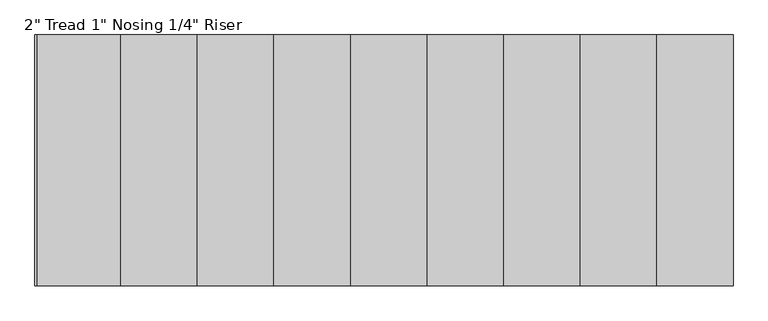
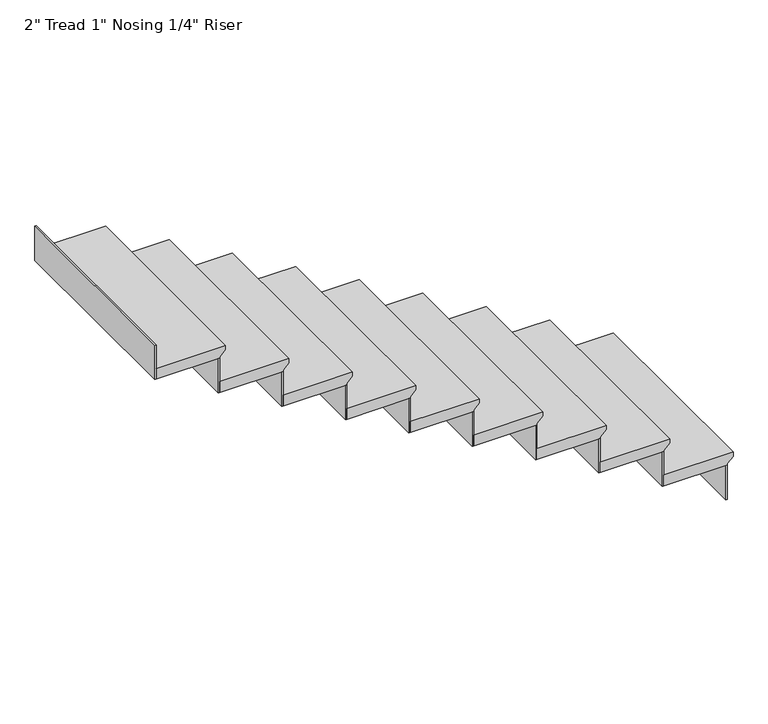
"""IFC4 building model written with IfcOpenShell, lengths in millimetres: stair flight geometry."""

from ifc_helpers import new_model, si_unit, frame, origin, place, context, project, spatial, polyline, outline, extrude, source, transform, mapped, element, save


def stair_flight_466e09e8(model_context):
    return source(origin(), model_context, "Body", "SweptSolid", [
        extrude(outline(polyline([(14561.82, 923.4845537), (14561.82, 618.6845537), (14511.02, 618.6845537), (14511.02, 898.0845537), (14517.37, 898.0845537), (14542.77, 923.4845537), (14561.82, 923.4845537)])), frame((0.0, -5753.3544725, 0.0), z_axis=(0.0, 1.0, 0.0), x_axis=(0.0, 0.0, 1.0)), (0.0, 0.0, 1.0), 914.4),
        extrude(outline(polyline([(891.7345537, -4838.9544725), (898.0845537, -4838.9544725), (898.0845537, -5753.3544725), (891.7345537, -5753.3544725), (891.7345537, -4838.9544725)])), frame((0.0, 0.0, 14351.0), z_axis=(0.0, 0.0, 1.0), x_axis=(1.0, 0.0, 0.0)), (0.0, 0.0, 1.0), 160.02),
        extrude(outline(polyline([(612.3345537, -4838.9544725), (618.6845537, -4838.9544725), (618.6845537, -5753.3544725), (612.3345537, -5753.3544725), (612.3345537, -4838.9544725)])), frame((0.0, 0.0, 14511.02), z_axis=(0.0, 0.0, 1.0), x_axis=(1.0, 0.0, 0.0)), (0.0, 0.0, 1.0), 160.02),
        extrude(outline(polyline([(14721.84, 644.0845537), (14721.84, 339.2845537), (14671.04, 339.2845537), (14671.04, 618.6845537), (14677.39, 618.6845537), (14702.79, 644.0845537), (14721.84, 644.0845537)])), frame((0.0, -5753.3544725, 0.0), z_axis=(0.0, 1.0, 0.0), x_axis=(0.0, 0.0, 1.0)), (0.0, 0.0, 1.0), 914.4),
        extrude(outline(polyline([(332.9345537, -4838.9544725), (339.2845537, -4838.9544725), (339.2845537, -5753.3544725), (332.9345537, -5753.3544725), (332.9345537, -4838.9544725)])), frame((0.0, 0.0, 14671.04), z_axis=(0.0, 0.0, 1.0), x_axis=(1.0, 0.0, 0.0)), (0.0, 0.0, 1.0), 160.02),
        extrude(outline(polyline([(14881.86, 364.6845537), (14881.86, 59.8845537), (14831.06, 59.8845537), (14831.06, 339.2845537), (14837.41, 339.2845537), (14862.81, 364.6845537), (14881.86, 364.6845537)])), frame((0.0, -5753.3544725, 0.0), z_axis=(0.0, 1.0, 0.0), x_axis=(0.0, 0.0, 1.0)), (0.0, 0.0, 1.0), 914.4),
        extrude(outline(polyline([(53.5345537, -4838.9544725), (59.8845537, -4838.9544725), (59.8845537, -5753.3544725), (53.5345537, -5753.3544725), (53.5345537, -4838.9544725)])), frame((0.0, 0.0, 14831.06), z_axis=(0.0, 0.0, 1.0), x_axis=(1.0, 0.0, 0.0)), (0.0, 0.0, 1.0), 160.02),
        extrude(outline(polyline([(15041.88, 85.2845537), (15041.88, -219.5154463), (14991.08, -219.5154463), (14991.08, 59.8845537), (14997.43, 59.8845537), (15022.83, 85.2845537), (15041.88, 85.2845537)])), frame((0.0, -5753.3544725, 0.0), z_axis=(0.0, 1.0, 0.0), x_axis=(0.0, 0.0, 1.0)), (0.0, 0.0, 1.0), 914.4),
        extrude(outline(polyline([(-225.8654463, -4838.9544725), (-219.5154463, -4838.9544725), (-219.5154463, -5753.3544725), (-225.8654463, -5753.3544725), (-225.8654463, -4838.9544725)])), frame((0.0, 0.0, 14991.08), z_axis=(0.0, 0.0, 1.0), x_axis=(1.0, 0.0, 0.0)), (0.0, 0.0, 1.0), 160.02),
        extrude(outline(polyline([(15201.9, -194.1154463), (15201.9, -498.9154463), (15151.1, -498.9154463), (15151.1, -219.5154463), (15157.45, -219.5154463), (15182.85, -194.1154463), (15201.9, -194.1154463)])), frame((0.0, -5753.3544725, 0.0), z_axis=(0.0, 1.0, 0.0), x_axis=(0.0, 0.0, 1.0)), (0.0, 0.0, 1.0), 914.4),
        extrude(outline(polyline([(-505.2654463, -4838.9544725), (-498.9154463, -4838.9544725), (-498.9154463, -5753.3544725), (-505.2654463, -5753.3544725), (-505.2654463, -4838.9544725)])), frame((0.0, 0.0, 15151.1), z_axis=(0.0, 0.0, 1.0), x_axis=(1.0, 0.0, 0.0)), (0.0, 0.0, 1.0), 160.02),
        extrude(outline(polyline([(15361.92, -473.5154463), (15361.92, -778.3154463), (15311.12, -778.3154463), (15311.12, -498.9154463), (15317.47, -498.9154463), (15342.87, -473.5154463), (15361.92, -473.5154463)])), frame((0.0, -5753.3544725, 0.0), z_axis=(0.0, 1.0, 0.0), x_axis=(0.0, 0.0, 1.0)), (0.0, 0.0, 1.0), 914.4),
        extrude(outline(polyline([(-784.6654463, -4838.9544725), (-778.3154463, -4838.9544725), (-778.3154463, -5753.3544725), (-784.6654463, -5753.3544725), (-784.6654463, -4838.9544725)])), frame((0.0, 0.0, 15311.12), z_axis=(0.0, 0.0, 1.0), x_axis=(1.0, 0.0, 0.0)), (0.0, 0.0, 1.0), 160.02),
        extrude(outline(polyline([(15521.94, -752.9154463), (15521.94, -1057.7154463), (15471.14, -1057.7154463), (15471.14, -778.3154463), (15477.49, -778.3154463), (15502.89, -752.9154463), (15521.94, -752.9154463)])), frame((0.0, -5753.3544725, 0.0), z_axis=(0.0, 1.0, 0.0), x_axis=(0.0, 0.0, 1.0)), (0.0, 0.0, 1.0), 914.4),
        extrude(outline(polyline([(-1064.0654463, -4838.9544725), (-1057.7154463, -4838.9544725), (-1057.7154463, -5753.3544725), (-1064.0654463, -5753.3544725), (-1064.0654463, -4838.9544725)])), frame((0.0, 0.0, 15471.14), z_axis=(0.0, 0.0, 1.0), x_axis=(1.0, 0.0, 0.0)), (0.0, 0.0, 1.0), 160.02),
        extrude(outline(polyline([(15681.96, -1032.3154463), (15681.96, -1337.1154463), (15631.16, -1337.1154463), (15631.16, -1057.7154463), (15637.51, -1057.7154463), (15662.91, -1032.3154463), (15681.96, -1032.3154463)])), frame((0.0, -5753.3544725, 0.0), z_axis=(0.0, 1.0, 0.0), x_axis=(0.0, 0.0, 1.0)), (0.0, 0.0, 1.0), 914.4),
        extrude(outline(polyline([(-1343.4654463, -4838.9544725), (-1337.1154463, -4838.9544725), (-1337.1154463, -5753.3544725), (-1343.4654463, -5753.3544725), (-1343.4654463, -4838.9544725)])), frame((0.0, 0.0, 15631.16), z_axis=(0.0, 0.0, 1.0), x_axis=(1.0, 0.0, 0.0)), (0.0, 0.0, 1.0), 160.02),
        extrude(outline(polyline([(-1622.8654463, -4838.9544725), (-1616.5154463, -4838.9544725), (-1616.5154463, -5753.3544725), (-1622.8654463, -5753.3544725), (-1622.8654463, -4838.9544725)])), frame((0.0, 0.0, 15791.18), z_axis=(0.0, 0.0, 1.0), x_axis=(1.0, 0.0, 0.0)), (0.0, 0.0, 1.0), 160.02),
        extrude(outline(polyline([(15841.98, -1311.7154463), (15841.98, -1616.5154463), (15791.18, -1616.5154463), (15791.18, -1337.1154463), (15797.53, -1337.1154463), (15822.93, -1311.7154463), (15841.98, -1311.7154463)])), frame((0.0, -5753.3544725, 0.0), z_axis=(0.0, 1.0, 0.0), x_axis=(0.0, 0.0, 1.0)), (0.0, 0.0, 1.0), 914.4),
    ])


if __name__ == "__main__":
    model = new_model("IFC4")
    model_context = context("Model", 3, world=origin())
    ifc_project = project(units=[si_unit("LENGTHUNIT", "METRE", prefix="MILLI")], contexts=[model_context])
    site = spatial("IfcSite", under=ifc_project)
    building = spatial("IfcBuilding", under=site)
    placement = place(None, origin())
    stair_flight_shape = stair_flight_466e09e8(model_context)
    element("IfcStairFlight", 1, ObjectType="2\" Tread 1\" Nosing 1/4\" Riser", at=placement, inside=building, context=model_context, shape_type="MappedRepresentation", body=[
        mapped(stair_flight_shape, transform((0.0, 0.0, 0.0), x_axis=(1.0, 0.0, 0.0), y_axis=(0.0, 1.0, 0.0), z_axis=(0.0, 0.0, 1.0))),
    ])
    save(model, "model.ifc")
